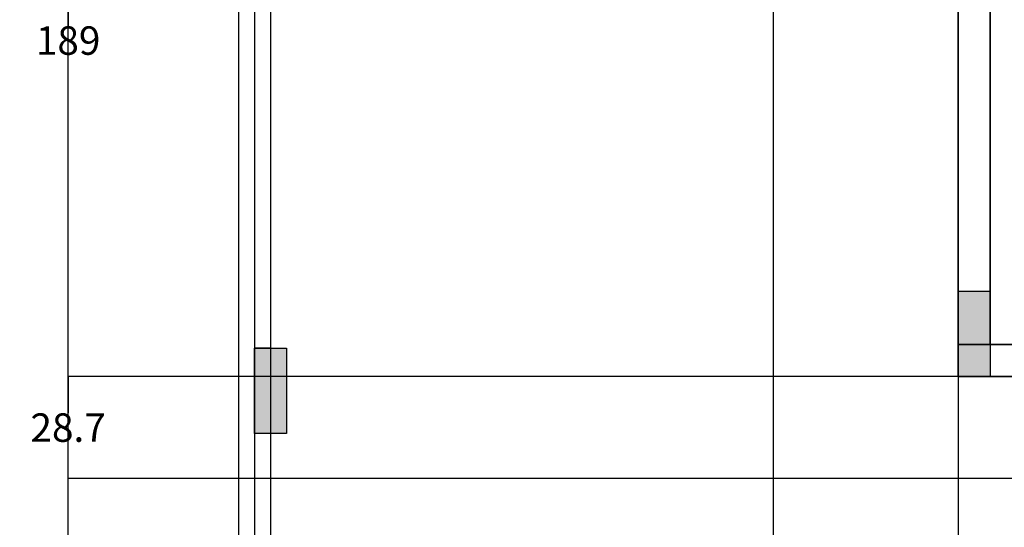
# Model space of a CAD drawing. Units: inches. Extents: x -48 to 50072, y 0 to 21068.
# Tile 58 of 75: x 697 to 974, y 517 to 660. Entities that reach past the tile are written whole.
import ezdxf

# ---------------------------------------------------------------- set-up
doc = ezdxf.new("R2010")
doc.units = ezdxf.units.IN
doc.header["$MEASUREMENT"] = 0
doc.linetypes.add('ACAD_ISO02W100', pattern=[15, 12, -3])
for name, color, linetype, lineweight in [('A-ANNO-DIMS', 2, 'Continuous', 18), ('A-COLS', 1, 'Continuous', 35), ('A-WALL', 7, 'Continuous', 35), ('C-PROP', 7, 'Continuous', 25), ('C-PROP-REF', 32, 'ACAD_ISO02W100', 13)]:
    doc.layers.add(name, color=color, linetype=linetype, lineweight=lineweight)
doc.styles.get("Standard").update_dxf_attribs({"font": 'arial.ttf'})
doc.dimstyles.get("Standard").update_dxf_attribs({"dimtxt": 8, "dimasz": 0.18, "dimexe": 0.18, "dimexo": 0.0625, "dimgap": 0.09, "dimtad": 0, "dimtih": 1, "dimtoh": 1, "dimdec": 1, "dimzin": 0, "dimdsep": 46, "dimlunit": 4, "dimtxsty": 'Standard', "dimblk": 'ARCHTICK', "dimcen": 0.09, "dimadec": 0, "dimazin": 0, "dimtfac": 1, "dimtdec": 1, "dimtofl": 0, "dimtmove": 0, "dimatfit": 3, "dimldrblk": 'ARCHTICK', "dimfxl": 1, "dimtolj": 1, "dimtzin": 0, "dimarcsym": 0})

# ---------------------------------------------------------------- blocks, each defined once
blk = doc.blocks.new('bnniku')
at = {"layer": 'Defpoints'}
h = blk.add_hatch(color=256, dxfattribs=at)
h.dxf.hatch_style = 1
h.paths.add_polyline_path([(767.55, 1114.04), (758.55, 1114.04), (758.55, 1090.04), (767.55, 1090.04)])
for p, q in [((758.55, 1114.04), (767.55, 1114.04)), ((758.55, 1090.04), (758.55, 1114.04)), ((767.55, 1114.04), (767.55, 1090.04)), ((767.55, 1090.04), (758.55, 1090.04))]:
    blk.add_line(p, q, dxfattribs=at)
blk = doc.blocks.new('_ArchTick')
at = {"color": 0, "linetype": 'ByBlock', "const_width": 0.15}
blk.add_lwpolyline([(-0.5, -0.5), (0.5, 0.5)], dxfattribs=at)
blk = doc.blocks.new('*D130')
at = {"layer": 'A-ANNO-DIMS', "color": 0, "lineweight": -2, "transparency": 16777216}
for p, q in [((758.7, 1241.46), (710.63, 1241.46)), ((710.81, 1241.46), (710.81, 767.29)), ((710.81, 284.76), (710.81, 758.94)), ((758.7, 284.76), (710.63, 284.76))]:
    blk.add_line(p, q, dxfattribs=at)
at = {"layer": 'Defpoints', "color": 0, "transparency": 16777216}
for p in [(710.81, 1241.46), (758.76, 1241.46), (758.76, 284.76)]:
    blk.add_point(p, dxfattribs=at)
at = {"layer": 'A-ANNO-DIMS', "color": 0, "lineweight": -2, "transparency": 16777216, "xscale": 0.18, "yscale": 0.18, "zscale": 0.18}
for p, rotation in [((710.81, 1241.46), 90), ((710.81, 284.76), 270)]:
    blk.add_blockref('_ArchTick', p, dxfattribs=dict(at, rotation=rotation))
at = {"layer": 'A-ANNO-DIMS', "color": 0, "transparency": 16777216, "insert": (710.81, 763.11), "char_height": 8, "attachment_point": 5}
blk.add_mtext('\\A1;956.7', dxfattribs=at)
blk = doc.blocks.new('*D135')
at = {"layer": 'A-ANNO-DIMS', "color": 0, "lineweight": -2, "transparency": 16777216}
for p, q in [((763.26, 748.4), (763.26, 236.63)), ((909.26, 748.4), (909.26, 236.63)), ((763.26, 236.81), (827.71, 236.81)), ((909.26, 236.81), (844.81, 236.81))]:
    blk.add_line(p, q, dxfattribs=at)
at = {"layer": 'Defpoints', "color": 0, "transparency": 16777216}
for p in [(763.26, 748.46), (909.26, 748.46), (909.26, 236.81)]:
    blk.add_point(p, dxfattribs=at)
at = {"layer": 'A-ANNO-DIMS', "color": 0, "lineweight": -2, "transparency": 16777216, "xscale": 0.18, "yscale": 0.18, "zscale": 0.18, "rotation": 180}
blk.add_blockref('_ArchTick', (763.26, 236.81), dxfattribs=at)
at = {"layer": 'A-ANNO-DIMS', "color": 0, "lineweight": -2, "transparency": 16777216, "xscale": 0.18, "yscale": 0.18, "zscale": 0.18}
blk.add_blockref('_ArchTick', (909.26, 236.81), dxfattribs=at)
at = {"layer": 'A-ANNO-DIMS', "color": 0, "transparency": 16777216, "insert": (836.26, 236.81), "char_height": 8, "attachment_point": 5}
blk.add_mtext('\\A1;146', dxfattribs=at)
blk = doc.blocks.new('*D136')
at = {"layer": 'A-ANNO-DIMS', "color": 0, "lineweight": -2, "transparency": 16777216}
for p, q in [((909.26, 748.4), (909.26, 236.63)), ((961.26, 559.4), (961.26, 236.63)), ((909.26, 236.81), (929.48, 236.81)), ((961.26, 236.81), (941.04, 236.81))]:
    blk.add_line(p, q, dxfattribs=at)
at = {"layer": 'Defpoints', "color": 0, "transparency": 16777216}
for p in [(909.26, 748.46), (961.26, 559.46), (961.26, 236.81)]:
    blk.add_point(p, dxfattribs=at)
at = {"layer": 'A-ANNO-DIMS', "color": 0, "lineweight": -2, "transparency": 16777216, "xscale": 0.18, "yscale": 0.18, "zscale": 0.18, "rotation": 180}
blk.add_blockref('_ArchTick', (909.26, 236.81), dxfattribs=at)
at = {"layer": 'A-ANNO-DIMS', "color": 0, "lineweight": -2, "transparency": 16777216, "xscale": 0.18, "yscale": 0.18, "zscale": 0.18}
blk.add_blockref('_ArchTick', (961.26, 236.81), dxfattribs=at)
at = {"layer": 'A-ANNO-DIMS', "color": 0, "transparency": 16777216, "insert": (935.26, 236.81), "char_height": 8, "attachment_point": 5}
blk.add_mtext('\\A1;52', dxfattribs=at)
blk = doc.blocks.new('*D137')
at = {"layer": 'A-ANNO-DIMS', "color": 0, "lineweight": -2, "transparency": 16777216}
for p, q in [((961.26, 559.4), (961.26, 236.63)), ((1042.26, 559.4), (1042.26, 236.63)), ((961.26, 236.81), (996.71, 236.81)), ((1042.26, 236.81), (1006.81, 236.81))]:
    blk.add_line(p, q, dxfattribs=at)
at = {"layer": 'Defpoints', "color": 0, "transparency": 16777216}
for p in [(961.26, 559.46), (1042.26, 559.46), (1042.26, 236.81)]:
    blk.add_point(p, dxfattribs=at)
at = {"layer": 'A-ANNO-DIMS', "color": 0, "lineweight": -2, "transparency": 16777216, "xscale": 0.18, "yscale": 0.18, "zscale": 0.18, "rotation": 180}
blk.add_blockref('_ArchTick', (961.26, 236.81), dxfattribs=at)
at = {"layer": 'A-ANNO-DIMS', "color": 0, "lineweight": -2, "transparency": 16777216, "xscale": 0.18, "yscale": 0.18, "zscale": 0.18}
blk.add_blockref('_ArchTick', (1042.26, 236.81), dxfattribs=at)
at = {"layer": 'A-ANNO-DIMS', "color": 0, "transparency": 16777216, "insert": (1001.76, 236.81), "char_height": 8, "attachment_point": 5}
blk.add_mtext('\\A1;81', dxfattribs=at)
blk = doc.blocks.new('*D145')
at = {"layer": 'A-ANNO-DIMS', "color": 0, "lineweight": -2, "transparency": 16777216}
for p, q in [((961.2, 748.46), (710.63, 748.46)), ((710.81, 748.46), (710.81, 658.14)), ((710.81, 559.46), (710.81, 649.79)), ((961.2, 559.46), (710.63, 559.46))]:
    blk.add_line(p, q, dxfattribs=at)
at = {"layer": 'Defpoints', "color": 0, "transparency": 16777216}
for p in [(710.81, 748.46), (961.26, 748.46), (961.26, 559.46)]:
    blk.add_point(p, dxfattribs=at)
at = {"layer": 'A-ANNO-DIMS', "color": 0, "lineweight": -2, "transparency": 16777216, "xscale": 0.18, "yscale": 0.18, "zscale": 0.18}
for p, rotation in [((710.81, 748.46), 90), ((710.81, 559.46), 270)]:
    blk.add_blockref('_ArchTick', p, dxfattribs=dict(at, rotation=rotation))
at = {"layer": 'A-ANNO-DIMS', "color": 0, "transparency": 16777216, "insert": (710.81, 653.96), "char_height": 8, "attachment_point": 5}
blk.add_mtext('\\A1;189', dxfattribs=at)
blk = doc.blocks.new('*D146')
at = {"layer": 'A-ANNO-DIMS', "color": 0, "lineweight": -2, "transparency": 16777216}
for p, q in [((1208.7, 559.46), (710.63, 559.46)), ((710.81, 559.46), (710.81, 549.29)), ((710.81, 530.76), (710.81, 540.94)), ((1208.7, 530.76), (710.63, 530.76))]:
    blk.add_line(p, q, dxfattribs=at)
at = {"layer": 'Defpoints', "color": 0, "transparency": 16777216}
for p in [(710.81, 559.46), (1208.76, 559.46), (1208.76, 530.76)]:
    blk.add_point(p, dxfattribs=at)
at = {"layer": 'A-ANNO-DIMS', "color": 0, "lineweight": -2, "transparency": 16777216, "xscale": 0.18, "yscale": 0.18, "zscale": 0.18}
for p, rotation in [((710.81, 559.46), 90), ((710.81, 530.76), 270)]:
    blk.add_blockref('_ArchTick', p, dxfattribs=dict(at, rotation=rotation))
at = {"layer": 'A-ANNO-DIMS', "color": 0, "transparency": 16777216, "insert": (710.81, 545.11), "char_height": 8, "attachment_point": 5}
blk.add_mtext('\\A1;28.7', dxfattribs=at)

msp = doc.modelspace()

# ---------------------------------------------------------------- linework, layer by layer
at = {"layer": 'A-WALL'}
for p, q in [((961.261, 559.464), (961.261, 748.464)), ((970.261, 568.464), (970.261, 691.464)), ((1208.761, 568.464), (961.261, 568.464)), ((763.261, 567.447), (767.761, 567.447)), ((1208.761, 559.464), (961.261, 559.464))]:
    msp.add_line(p, q, dxfattribs=at)
at = {"layer": 'C-PROP'}
for p, q in [((758.761, 1241.464), (758.761, 284.764)), ((767.761, 931.464), (767.761, 293.764))]:
    msp.add_line(p, q, dxfattribs=at)
at = {"layer": 'C-PROP-REF'}
msp.add_line((763.261, 1236.964), (763.261, 284.764), dxfattribs=at)

# ---------------------------------------------------------------- block references
at = {"layer": 'A-COLS'}
for p in [(202.709, -530.573), (4.709, -546.59)]:
    msp.add_blockref('bnniku', p, dxfattribs=at)

# ---------------------------------------------------------------- dimensions: what is measured, and where the dimension line sits
at = {"layer": 'A-ANNO-DIMS'}
for base, p1, p2, override, picture, middle in [((710.811, 1241.464), (758.761, 284.764), (758.761, 1241.464), {"dimdec": 1, "dimlfac": 1, "dimrnd": 0, "dimzin": 0, "dimdsep": 46, "dimlunit": 2}, '*D130', (710.811, 763.114)), ((710.811, 748.464), (961.261, 559.464), (961.261, 748.464), {"dimdec": 0, "dimlfac": 1, "dimrnd": 0, "dimzin": 0, "dimdsep": 46, "dimlunit": 2}, '*D145', (710.811, 653.964)), ((710.811, 559.464), (1208.761, 530.764), (1208.761, 559.464), {"dimdec": 1, "dimlfac": 1, "dimrnd": 0, "dimzin": 0, "dimdsep": 46, "dimlunit": 2}, '*D146', (710.811, 545.114))]:
    dim = msp.add_linear_dim(base=base, p1=p1, p2=p2, angle=90, dimstyle='Standard', override=override, dxfattribs=at)
    dim.commit()
    dim.dimension.update_dxf_attribs({"geometry": picture, "text_midpoint": middle})
for base, p1, p2, picture, middle in [((909.261, 236.814), (763.261, 748.464), (909.261, 748.464), '*D135', (836.261, 236.814)), ((961.261, 236.814), (909.261, 748.464), (961.261, 559.464), '*D136', (935.261, 236.814)), ((1042.261, 236.814), (961.261, 559.464), (1042.261, 559.464), '*D137', (1001.761, 236.814))]:
    dim = msp.add_linear_dim(base=base, p1=p1, p2=p2, dimstyle='Standard', override={"dimdec": 0, "dimlfac": 1, "dimrnd": 0, "dimzin": 0, "dimdsep": 46, "dimlunit": 2}, dxfattribs=at)
    dim.commit()
    dim.dimension.update_dxf_attribs({"geometry": picture, "text_midpoint": middle})

doc.saveas('drawing.dxf')
